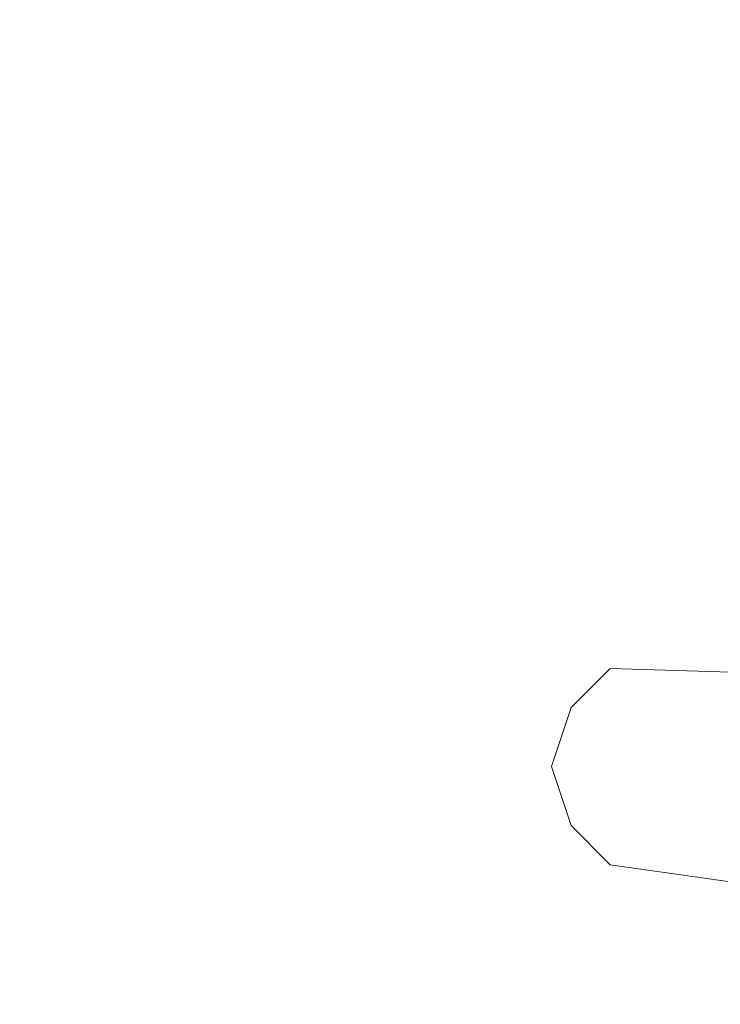
# Model space of a CAD drawing. Units: inches. Extents: x 375 to 1122, y 27 to 1069.
# Tile 61 of 155: x 732.625 to 734.823, y 308.498 to 311.585. Entities that reach past the tile are written whole.
import ezdxf

# ---------------------------------------------------------------- set-up
doc = ezdxf.new("R2010")
doc.units = ezdxf.units.IN
doc.layers.add('A-ANNO-DIMS', color=2, linetype='Continuous', lineweight=18)
doc.layers.add('Furniture', color=30, linetype='Continuous', lineweight=18)
doc.styles.get("Standard").update_dxf_attribs({"font": 'arial.ttf'})
doc.dimstyles.new('ISO-25', dxfattribs={"dimtxt": 12, "dimasz": 2.5, "dimexe": 1.5, "dimexo": 1.5, "dimtad": 1, "dimdec": 1, "dimlunit": 3, "dimtxsty": 'Standard', "dimblk": 'ARCHTICK', "dimcen": 2.5, "dimadec": 0, "dimazin": 0, "dimtfac": 1, "dimtdec": 1, "dimtmove": 0, "dimatfit": 3, "dimfxl": 1.5, "dimfxlon": 1, "dimarcsym": 0})

# ---------------------------------------------------------------- blocks, each defined once
blk = doc.blocks.new('A$C403C54AD')
for points, invisible_edges in [([(0.933982, 1.238319, -0.039653), (0.91859, 1.238319, -0.039653), (0.920129, 1.287573, -0.039653), (0.935521, 1.249093, -0.039653)], 5), ([(0.933982, 1.238319, -0.041193), (0.91859, 1.238319, -0.041193), (0.920129, 1.287573, -0.041193), (0.935521, 1.249093, -0.041193)], 5), ([(0.920129, 1.287573, -0.041193), (0.920129, 1.287573, -0.039653), (0.91859, 1.238319, -0.039653), (0.91859, 1.238319, -0.041193)], 5), ([(0.933982, 1.238319, -0.039653), (0.933982, 1.238319, -0.041193), (0.935521, 1.249093, -0.041193), (0.935521, 1.249093, -0.039653)], 5), ([(0.921668, 1.23524, -0.039653), (0.930903, 1.23524, -0.039653), (0.933982, 1.238319, -0.039653), (0.91859, 1.238319, -0.039653)], 5), ([(0.921668, 1.23524, -0.041193), (0.930903, 1.23524, -0.041193), (0.933982, 1.238319, -0.041193), (0.91859, 1.238319, -0.041193)], 5), ([(0.91859, 1.238319, -0.039653), (0.91859, 1.238319, -0.041193), (0.921668, 1.23524, -0.041193), (0.921668, 1.23524, -0.039653)], 5), ([(0.930903, 1.23524, -0.041193), (0.930903, 1.23524, -0.039653), (0.933982, 1.238319, -0.039653), (0.933982, 1.238319, -0.041193)], 5), ([(0.926286, 1.233701, -0.039653), (0.926286, 1.233701, -0.039653), (0.921668, 1.23524, -0.039653), (0.930903, 1.23524, -0.039653)], 4), ([(0.926286, 1.233701, -0.041193), (0.926286, 1.233701, -0.041193), (0.921668, 1.23524, -0.041193), (0.930903, 1.23524, -0.041193)], 4), ([(0.921668, 1.23524, -0.041193), (0.921668, 1.23524, -0.039653), (0.926286, 1.233701, -0.039653), (0.926286, 1.233701, -0.041193)], 1), ([(0.926286, 1.233701, -0.039653), (0.926286, 1.233701, -0.041193), (0.930903, 1.23524, -0.041193), (0.930903, 1.23524, -0.039653)], 4)]:
    blk.add_3dface(points, dxfattribs=dict(invisible_edges=invisible_edges))
blk = doc.blocks.new('_ArchTick')
at = {"color": 0, "linetype": 'ByBlock', "const_width": 0.15}
blk.add_lwpolyline([(-0.5, -0.5), (0.5, 0.5)], dxfattribs=at)
blk = doc.blocks.new('*D94')
at = {"layer": 'A-ANNO-DIMS', "color": 0, "lineweight": -2, "transparency": 16777216}
for p, q in [((734.0073, 117.5277), (734.0073, 114.5277)), ((773.0073, 117.5277), (773.0073, 114.5277)), ((734.0073, 116.0277), (773.0073, 116.0277))]:
    blk.add_line(p, q, dxfattribs=at)
at = {"layer": 'Defpoints', "color": 0, "transparency": 16777216}
for p in [(734.0073, 667.5277), (773.0073, 667.5277), (773.0073, 116.0277)]:
    blk.add_point(p, dxfattribs=at)
at = {"layer": 'A-ANNO-DIMS', "color": 0, "lineweight": -2, "transparency": 16777216, "xscale": 2.5, "yscale": 2.5, "zscale": 2.5, "rotation": 180}
blk.add_blockref('_ArchTick', (734.0073, 116.0277), dxfattribs=at)
at = {"layer": 'A-ANNO-DIMS', "color": 0, "lineweight": -2, "transparency": 16777216, "xscale": 2.5, "yscale": 2.5, "zscale": 2.5}
blk.add_blockref('_ArchTick', (773.0073, 116.0277), dxfattribs=at)
at = {"layer": 'A-ANNO-DIMS', "color": 0, "transparency": 16777216, "insert": (753.5073, 122.7837), "char_height": 12, "attachment_point": 5}
blk.add_mtext('3\'-3"', dxfattribs=at)

msp = doc.modelspace()

# ---------------------------------------------------------------- block references
at = {"layer": 'Furniture', "xscale": 39.9918517141215, "yscale": 39.9918517141215, "zscale": 39.9918517141215, "rotation": 270}
msp.add_blockref('A$C403C54AD', (684.9549, 346.2875, 0.024), dxfattribs=at)

# ---------------------------------------------------------------- dimensions: what is measured, and where the dimension line sits
at = {"layer": 'A-ANNO-DIMS'}
dim = msp.add_linear_dim(base=(773.0073, 116.0277), p1=(734.0073, 667.5277), p2=(773.0073, 667.5277), dimstyle='ISO-25', override={"dimdec": 1, "dimlfac": 1, "dimrnd": 0, "dimzin": 1, "dimdsep": 46, "dimlunit": 4, "dimfrac": 2}, dxfattribs=at)
dim.commit()
dim.dimension.update_dxf_attribs({"geometry": '*D94', "text_midpoint": (753.5073, 122.7837)})

doc.saveas('drawing.dxf')
